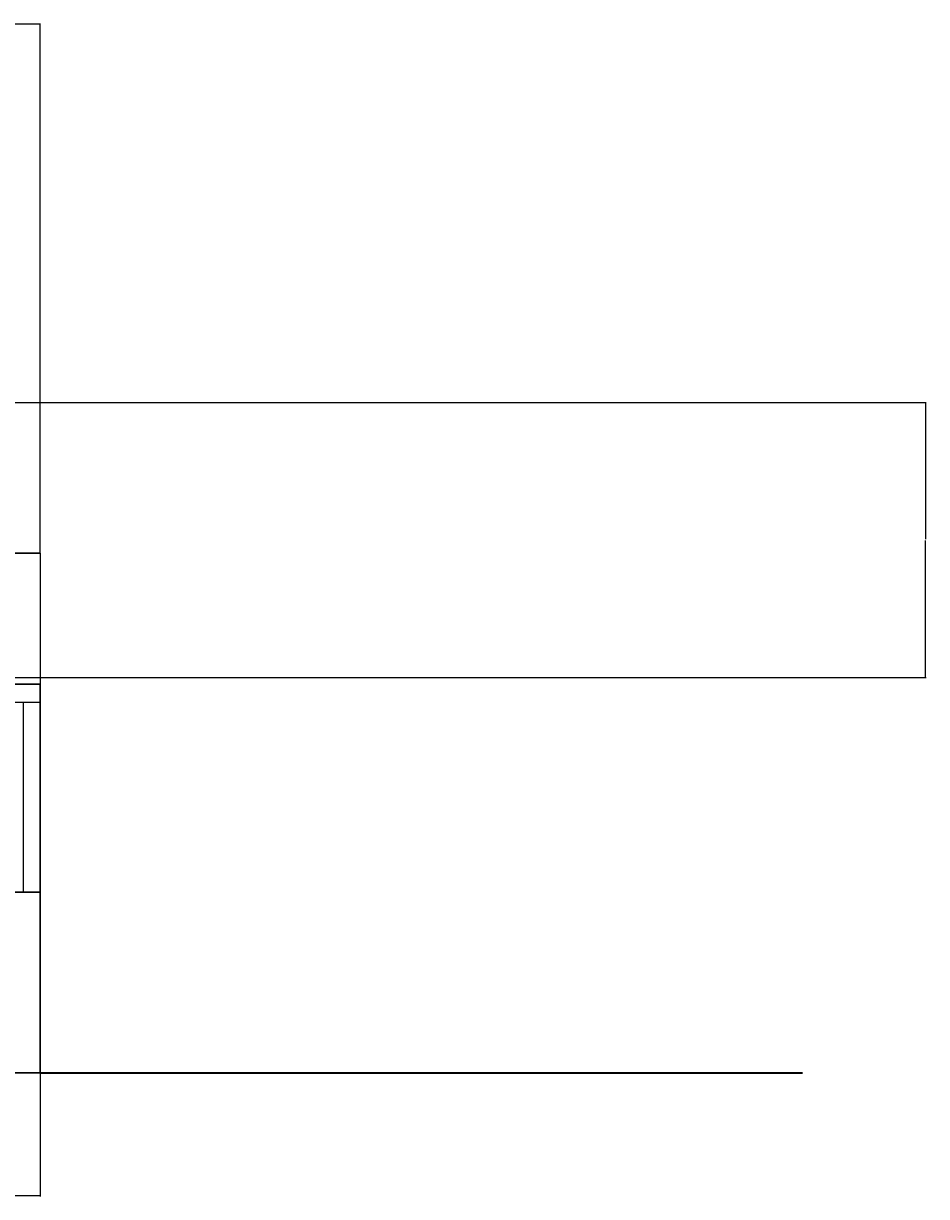
# Model space of a CAD drawing. Units: inches. Extents: x -14 to 886, y 45 to 435.
# Tile 5 of 5: x 586 to 886, y 45 to 435. Entities that reach past the tile are written whole.
import ezdxf

# ---------------------------------------------------------------- set-up
doc = ezdxf.new("R2010")
doc.units = ezdxf.units.IN
doc.header["$MEASUREMENT"] = 0
for name, color, linetype, lineweight in [('A-ANNO-DIMS', 2, 'Continuous', 18), ('A-WALL', 7, 'Continuous', 25), ('C-TOPO', 7, 'Continuous', 35), ('L-WALL', 7, 'Continuous', 30)]:
    doc.layers.add(name, color=color, linetype=linetype, lineweight=lineweight)
doc.styles.get("Standard").update_dxf_attribs({"font": 'arial.ttf'})
doc.dimstyles.get("Standard").update_dxf_attribs({"dimtxt": 0.18, "dimasz": 0.18, "dimexe": 0.18, "dimexo": 0.0625, "dimgap": 0.09, "dimtad": 0, "dimtih": 1, "dimtoh": 1, "dimdec": 4, "dimzin": 0, "dimdsep": 46, "dimtxsty": 'Standard', "dimcen": 0.09, "dimadec": 0, "dimazin": 0, "dimtfac": 1, "dimtdec": 4, "dimtofl": 0, "dimtmove": 0, "dimatfit": 3, "dimfxl": 1, "dimtolj": 1, "dimtzin": 0, "dimarcsym": 0})

# ---------------------------------------------------------------- blocks, each defined once
blk = doc.blocks.new('*D16')
at = {"layer": 'A-ANNO-DIMS', "color": 0, "lineweight": -2, "transparency": 16777216}
for p, q in [((111.3, 86.48), (111.3, 45.47)), ((591.3, 86.48), (591.3, 45.47)), ((111.48, 45.65), (351.01, 45.65)), ((591.12, 45.65), (351.59, 45.65))]:
    blk.add_line(p, q, dxfattribs=at)
at = {"layer": 'A-ANNO-DIMS', "color": 0, "transparency": 16777216}
for points in [[(111.48, 45.68), (111.48, 45.62), (111.3, 45.65)], [(591.12, 45.68), (591.12, 45.62), (591.3, 45.65)]]:
    blk.add_solid(points, dxfattribs=at)
at = {"layer": 'Defpoints', "color": 0, "transparency": 16777216}
for p in [(111.3, 86.54), (591.3, 86.54), (591.3, 45.65)]:
    blk.add_point(p, dxfattribs=at)
at = {"layer": 'A-ANNO-DIMS', "color": 0, "transparency": 16777216, "insert": (351.3, 45.65), "char_height": 0.18, "attachment_point": 5}
blk.add_mtext('\\A1;480', dxfattribs=at)
blk = doc.blocks.new('*D40')
at = {"layer": 'A-ANNO-DIMS', "color": 0, "lineweight": -2, "transparency": 16777216}
for p, q in [((537.25, 259.21), (537.25, 435.05)), ((537.43, 434.87), (563.88, 434.87)), ((591.12, 434.87), (564.67, 434.87)), ((591.3, 259.21), (591.3, 435.05))]:
    blk.add_line(p, q, dxfattribs=at)
at = {"layer": 'A-ANNO-DIMS', "color": 0, "transparency": 16777216}
for points in [[(537.43, 434.9), (537.43, 434.84), (537.25, 434.87)], [(591.12, 434.9), (591.12, 434.84), (591.3, 434.87)]]:
    blk.add_solid(points, dxfattribs=at)
at = {"layer": 'Defpoints', "color": 0, "transparency": 16777216}
for p in [(591.3, 434.87), (537.25, 259.14), (591.3, 259.14)]:
    blk.add_point(p, dxfattribs=at)
at = {"layer": 'A-ANNO-DIMS', "color": 0, "transparency": 16777216, "insert": (564.28, 434.87), "char_height": 0.18, "attachment_point": 5}
blk.add_mtext('\\A1;54.05', dxfattribs=at)
blk = doc.blocks.new('*D41')
at = {"layer": 'A-ANNO-DIMS', "color": 0, "lineweight": -2, "transparency": 16777216}
for p, q in [((591.24, 259.14), (-13.96, 259.14)), ((-13.78, 258.96), (-13.78, 203.02)), ((-13.78, 146.72), (-13.78, 202.66)), ((537.19, 146.54), (-13.96, 146.54))]:
    blk.add_line(p, q, dxfattribs=at)
at = {"layer": 'A-ANNO-DIMS', "color": 0, "transparency": 16777216}
for points in [[(-13.81, 258.96), (-13.75, 258.96), (-13.78, 259.14)], [(-13.81, 146.72), (-13.75, 146.72), (-13.78, 146.54)]]:
    blk.add_solid(points, dxfattribs=at)
at = {"layer": 'Defpoints', "color": 0, "transparency": 16777216}
for p in [(-13.78, 259.14), (591.3, 259.14), (537.25, 146.54)]:
    blk.add_point(p, dxfattribs=at)
at = {"layer": 'A-ANNO-DIMS', "color": 0, "transparency": 16777216, "insert": (-13.78, 202.84), "char_height": 0.18, "attachment_point": 5}
blk.add_mtext('\\A1;112.6', dxfattribs=at)
blk = doc.blocks.new('*D51')
at = {"layer": 'A-ANNO-DIMS', "color": 0, "lineweight": -2, "transparency": 16777216}
for p, q in [((370.91, 309.22), (885.58, 309.22)), ((885.4, 309.04), (885.4, 263.74)), ((885.4, 218.06), (885.4, 263.37)), ((370.91, 217.88), (885.58, 217.88))]:
    blk.add_line(p, q, dxfattribs=at)
at = {"layer": 'A-ANNO-DIMS', "color": 0, "transparency": 16777216}
for points in [[(885.37, 309.04), (885.43, 309.04), (885.4, 309.22)], [(885.37, 218.06), (885.43, 218.06), (885.4, 217.88)]]:
    blk.add_solid(points, dxfattribs=at)
at = {"layer": 'Defpoints', "color": 0, "transparency": 16777216}
for p in [(370.85, 309.22), (885.4, 309.22), (370.85, 217.88)]:
    blk.add_point(p, dxfattribs=at)
at = {"layer": 'A-ANNO-DIMS', "color": 0, "transparency": 16777216, "insert": (885.4, 263.55), "char_height": 0.18, "attachment_point": 5}
blk.add_mtext('\\A1;91.34', dxfattribs=at)

msp = doc.modelspace()

# ---------------------------------------------------------------- linework, layer by layer
at = {"layer": 'A-WALL'}
msp.add_line((537.2506, 215.6038), (591.3024, 215.6038), dxfattribs=at)
msp.add_lwpolyline([(591.3024, 215.6038), (537.2506, 215.6038), (537.2506, 259.1435), (591.3024, 259.1435)], close=True, dxfattribs=at)
msp.add_lwpolyline([(585.6689, 209.6038), (585.6689, 146.5389), (537.2506, 146.5389), (537.2506, 209.6038), (591.3024, 209.6038)], dxfattribs=at)
at = {"layer": 'C-TOPO'}
msp.add_line((591.3024, 86.5389), (844.511, 86.5389), dxfattribs=at)
at = {"layer": 'L-WALL'}
for p, q in [((591.3024, 215.6038), (591.3024, 86.5389)), ((591.3024, 146.5389), (391.7908, 146.5389)), ((591.3024, 86.5389), (379.7908, 86.5389))]:
    msp.add_line(p, q, dxfattribs=at)

# ---------------------------------------------------------------- dimensions: what is measured, and where the dimension line sits
at = {"layer": 'A-ANNO-DIMS'}
for base, p1, p2, override, picture, middle in [((591.3024, 434.8697), (537.2506, 259.1435), (591.3024, 259.1435), {"dimdec": 2, "dimlfac": 1, "dimrnd": 0, "dimzin": 0, "dimdsep": 46, "dimlunit": 2}, '*D40', (564.2765, 434.8697)), ((591.3024, 45.6489), (111.3024, 86.5389), (591.3024, 86.5389), {"dimdec": 0, "dimlfac": 1, "dimrnd": 0, "dimzin": 0, "dimdsep": 46, "dimlunit": 2}, '*D16', (351.3024, 45.6489))]:
    dim = msp.add_linear_dim(base=base, p1=p1, p2=p2, dimstyle='Standard', override=override, dxfattribs=at)
    dim.commit()
    dim.dimension.update_dxf_attribs({"geometry": picture, "text_midpoint": middle})
for base, p1, p2, override, picture, middle in [((885.401, 309.2241), (370.8507, 217.8839), (370.8507, 309.2241), {"dimdec": 2, "dimlfac": 1, "dimrnd": 0, "dimzin": 0, "dimdsep": 46, "dimlunit": 2}, '*D51', (885.401, 263.554)), ((-13.7769, 259.1435), (537.2506, 146.5389), (591.3024, 259.1435), {"dimdec": 1, "dimlfac": 1, "dimrnd": 0, "dimzin": 0, "dimdsep": 46, "dimlunit": 2}, '*D41', (-13.7769, 202.8412))]:
    dim = msp.add_linear_dim(base=base, p1=p1, p2=p2, angle=90, dimstyle='Standard', override=override, dxfattribs=at)
    dim.commit()
    dim.dimension.update_dxf_attribs({"geometry": picture, "text_midpoint": middle})

doc.saveas('drawing.dxf')
